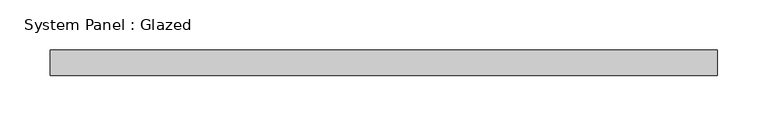
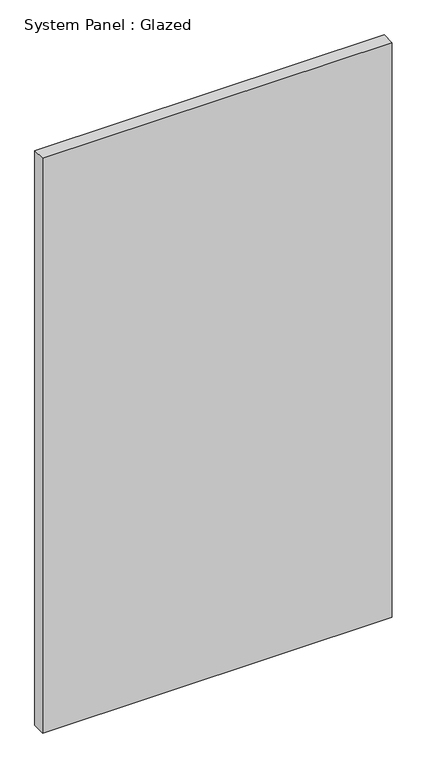
"""IFC4 building model written with IfcOpenShell, lengths in millimetres: plate geometry, System Panel : Glazed."""

from ifc_helpers import new_model, si_unit, origin, origin_with_axes, place, context, project, spatial, polyline, outline, extrude, source, transform, mapped, element, save


def system_panel_glazed_f0dacc13(model_context):
    return source(origin(), model_context, "Body", "SweptSolid", [
        extrude(outline(polyline([(332.5697385, 19.05), (-332.5697385, 19.05), (-332.5697385, 44.45), (332.5697385, 44.45), (332.5697385, 19.05)])), origin_with_axes(), (0.0, 0.0, 1.0), 1155.7),
    ])


if __name__ == "__main__":
    model = new_model("IFC4")
    model_context = context("Model", 3, world=origin())
    ifc_project = project(units=[si_unit("LENGTHUNIT", "METRE", prefix="MILLI")], contexts=[model_context])
    site = spatial("IfcSite", under=ifc_project)
    building = spatial("IfcBuilding", under=site)
    placement = place(None, origin())
    system_panel_glazed_shape = system_panel_glazed_f0dacc13(model_context)
    element("IfcPlate", 1, ObjectType="System Panel : Glazed", at=placement, inside=building, context=model_context, shape_type="MappedRepresentation", body=[
        mapped(system_panel_glazed_shape, transform((0.0, 0.0, 0.0), x_axis=(1.0, 0.0, 0.0), y_axis=(0.0, 1.0, 0.0), z_axis=(0.0, 0.0, 1.0))),
    ])
    save(model, "model.ifc")

# Revit data of these elements
# Type "System Panel : Glazed"
#   Construction Type Id = "GSP4R"
#   Analytic Construction = "1/8 in Pilkington single glazing"
#   Visual Light Transmittance = 0.9
#   Solar Heat Gain Coefficient = 0.86
#   Heat Transfer Coefficient (U) = 1.18115 BTU/(h·ft²·°F)
# Element 1 (IfcPlate, "System Panel : Glazed")
#   Materials on its faces: "Glass"
# Materials
#   "Glass": class "Glass", colour RGB 0 128 192, transparency 0.75, Description = "Soda Lime Glass", Cost = 0
